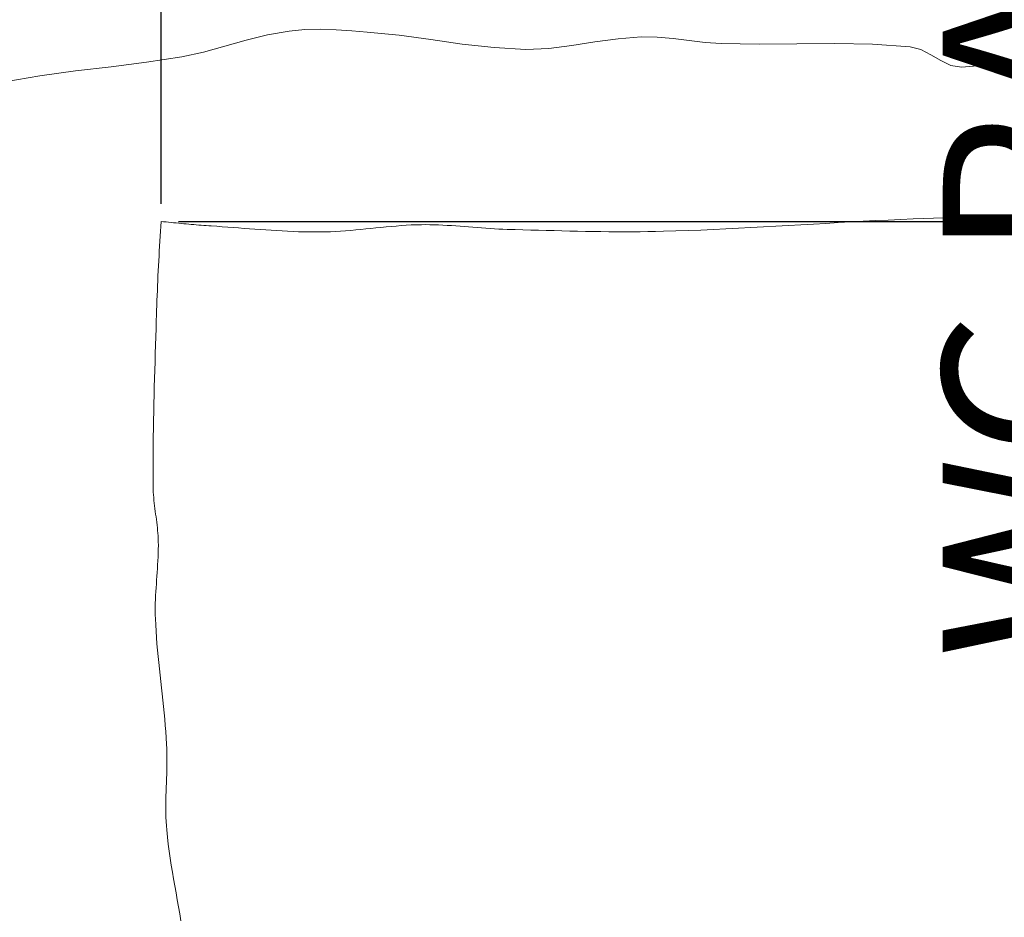
# Model space of a CAD drawing. Units: inches. Extents: x 2656 to 9931, y 1941 to 3068.
# Tile 19 of 46: x 2896 to 2932, y 2498 to 2530. Entities that reach past the tile are written whole.
import ezdxf

# ---------------------------------------------------------------- set-up
doc = ezdxf.new("R2010")
doc.units = ezdxf.units.IN
doc.layers.add('A-ANNO-DIMS', color=2, linetype='Continuous', lineweight=18)
doc.layers.add('A-FURN', color=8, linetype='Continuous', lineweight=13)
doc.styles.get("Standard").update_dxf_attribs({"font": 'arial.ttf'})
doc.dimstyles.new('ISO-25', dxfattribs={"dimtxt": 6, "dimasz": 2.5, "dimexe": 1.25, "dimexo": 0.625, "dimtad": 1, "dimdec": 0, "dimlunit": 3, "dimtxsty": 'Standard', "dimcen": 2.5, "dimadec": 0, "dimazin": 0, "dimtfac": 1, "dimtdec": 0, "dimtmove": 0, "dimatfit": 3, "dimfxl": 1, "dimarcsym": 0})

# ---------------------------------------------------------------- blocks, each defined once
blk = doc.blocks.new('BED-DOUBLE')
for p, q in [((27.981, 62.21), (27.218, 62.019)), ((28.754, 62.35), (27.981, 62.21)), ((29.308, 62.401), (28.754, 62.35)), ((29.865, 62.411), (29.308, 62.401)), ((30.423, 62.394), (29.865, 62.411)), ((30.981, 62.358), (30.423, 62.394)), ((31.538, 62.315), (30.981, 62.358)), ((32.669, 62.198), (31.538, 62.315)), ((33.797, 62.044), (32.669, 62.198)), ((41.299, 62.14), (40.475, 62.076)), ((41.872, 62.129), (41.299, 62.14)), ((42.443, 62.078), (41.872, 62.129)), ((26.459, 61.805), (25.698, 61.6)), ((27.218, 62.019), (26.459, 61.805)), ((34.924, 61.887), (33.797, 62.044)), ((36.054, 61.76), (34.924, 61.887)), ((38.833, 61.831), (38.012, 61.729)), ((39.653, 61.96), (38.833, 61.831)), ((40.475, 62.076), (39.653, 61.96)), ((43.013, 62.008), (42.443, 62.078)), ((43.584, 61.942), (43.013, 62.008)), ((44.157, 61.901), (43.584, 61.942)), ((45.504, 61.879), (44.157, 61.901)), ((46.854, 61.889), (45.504, 61.879)), ((48.203, 61.9), (46.854, 61.889)), ((49.55, 61.878), (48.203, 61.9)), ((50.893, 61.79), (49.55, 61.878)), ((51.27, 61.688), (50.893, 61.79)), ((24.929, 61.432), (23.668, 61.237)), ((25.698, 61.6), (24.929, 61.432)), ((37.187, 61.697), (36.054, 61.76)), ((38.012, 61.729), (37.187, 61.697)), ((51.627, 61.503), (51.27, 61.688)), ((51.978, 61.295), (51.627, 61.503)), ((22.401, 61.078), (21.133, 60.928)), ((23.668, 61.237), (22.401, 61.078)), ((52.336, 61.127), (51.978, 61.295)), ((52.714, 61.061), (52.336, 61.127)), ((53.7, 61.143), (52.714, 61.061)), ((54.677, 61.321), (53.7, 61.143)), ((19.868, 60.758), (18.612, 60.54)), ((21.133, 60.928), (19.868, 60.758)), ((24.187, 55.565), (24.175, 55.389)), ((24.276, 55.555), (24.187, 55.565)), ((24.366, 55.545), (24.276, 55.555)), ((24.455, 55.535), (24.366, 55.545)), ((24.544, 55.526), (24.455, 55.535)), ((24.634, 55.517), (24.544, 55.526)), ((24.723, 55.508), (24.634, 55.517)), ((24.813, 55.499), (24.723, 55.508)), ((24.902, 55.49), (24.813, 55.499)), ((24.992, 55.482), (24.902, 55.49)), ((25.081, 55.473), (24.992, 55.482)), ((25.171, 55.465), (25.081, 55.473)), ((25.26, 55.457), (25.171, 55.465)), ((47.438, 55.469), (46.993, 55.443)), ((47.883, 55.495), (47.438, 55.469)), ((48.328, 55.521), (47.883, 55.495)), ((48.773, 55.545), (48.328, 55.521)), ((49.218, 55.569), (48.773, 55.545)), ((49.663, 55.592), (49.218, 55.569)), ((50.109, 55.613), (49.663, 55.592)), ((50.554, 55.633), (50.109, 55.613)), ((50.999, 55.651), (50.554, 55.633)), ((51.36, 55.665), (50.999, 55.651)), ((51.72, 55.679), (51.36, 55.665)), ((52.081, 55.693), (51.72, 55.679)), ((52.441, 55.706), (52.081, 55.693)), ((52.802, 55.72), (52.441, 55.706)), ((53.162, 55.733), (52.802, 55.72)), ((53.522, 55.745), (53.162, 55.733)), ((53.883, 55.757), (53.522, 55.745)), ((54.244, 55.769), (53.883, 55.757)), ((54.604, 55.779), (54.244, 55.769)), ((24.164, 55.213), (24.153, 55.037)), ((24.175, 55.389), (24.164, 55.213)), ((25.35, 55.45), (25.26, 55.457)), ((25.439, 55.442), (25.35, 55.45)), ((25.529, 55.435), (25.439, 55.442)), ((25.619, 55.428), (25.529, 55.435)), ((25.708, 55.422), (25.619, 55.428)), ((25.798, 55.415), (25.708, 55.422)), ((25.888, 55.409), (25.798, 55.415)), ((25.977, 55.403), (25.888, 55.409)), ((26.172, 55.39), (25.977, 55.403)), ((26.366, 55.376), (26.172, 55.39)), ((26.56, 55.361), (26.366, 55.376)), ((26.754, 55.347), (26.56, 55.361)), ((26.949, 55.332), (26.754, 55.347)), ((27.143, 55.317), (26.949, 55.332)), ((27.337, 55.302), (27.143, 55.317)), ((27.531, 55.288), (27.337, 55.302)), ((27.726, 55.274), (27.531, 55.288)), ((27.92, 55.26), (27.726, 55.274)), ((28.114, 55.248), (27.92, 55.26)), ((28.309, 55.236), (28.114, 55.248)), ((28.503, 55.225), (28.309, 55.236)), ((28.698, 55.215), (28.503, 55.225)), ((28.892, 55.206), (28.698, 55.215)), ((29.087, 55.199), (28.892, 55.206)), ((29.281, 55.194), (29.087, 55.199)), ((29.476, 55.19), (29.281, 55.194)), ((29.67, 55.188), (29.476, 55.19)), ((29.865, 55.188), (29.67, 55.188)), ((30.045, 55.191), (29.865, 55.188)), ((30.226, 55.197), (30.045, 55.191)), ((30.406, 55.205), (30.226, 55.197)), ((30.586, 55.216), (30.406, 55.205)), ((30.766, 55.229), (30.586, 55.216)), ((30.946, 55.244), (30.766, 55.229)), ((31.126, 55.261), (30.946, 55.244)), ((31.306, 55.278), (31.126, 55.261)), ((31.486, 55.296), (31.306, 55.278)), ((31.665, 55.314), (31.486, 55.296)), ((31.845, 55.333), (31.665, 55.314)), ((32.025, 55.351), (31.845, 55.333)), ((32.205, 55.369), (32.025, 55.351)), ((32.385, 55.386), (32.205, 55.369)), ((32.565, 55.401), (32.385, 55.386)), ((32.745, 55.415), (32.565, 55.401)), ((32.925, 55.427), (32.745, 55.415)), ((33.105, 55.437), (32.925, 55.427)), ((33.285, 55.444), (33.105, 55.437)), ((33.466, 55.448), (33.285, 55.444)), ((33.619, 55.449), (33.466, 55.448)), ((33.772, 55.447), (33.619, 55.449)), ((33.926, 55.444), (33.772, 55.447)), ((34.079, 55.439), (33.926, 55.444)), ((34.232, 55.432), (34.079, 55.439)), ((34.385, 55.424), (34.232, 55.432)), ((34.538, 55.414), (34.385, 55.424)), ((34.691, 55.404), (34.538, 55.414)), ((34.844, 55.392), (34.691, 55.404)), ((34.997, 55.381), (34.844, 55.392)), ((35.15, 55.369), (34.997, 55.381)), ((35.303, 55.356), (35.15, 55.369)), ((35.456, 55.344), (35.303, 55.356)), ((35.609, 55.333), (35.456, 55.344)), ((35.762, 55.322), (35.609, 55.333)), ((35.915, 55.311), (35.762, 55.322)), ((36.068, 55.302), (35.915, 55.311)), ((36.221, 55.294), (36.068, 55.302)), ((36.374, 55.287), (36.221, 55.294)), ((36.528, 55.282), (36.374, 55.287)), ((36.806, 55.274), (36.528, 55.282)), ((37.084, 55.266), (36.806, 55.274)), ((37.362, 55.258), (37.084, 55.266)), ((37.641, 55.25), (37.362, 55.258)), ((37.919, 55.243), (37.641, 55.25)), ((38.198, 55.235), (37.919, 55.243)), ((38.476, 55.228), (38.198, 55.235)), ((38.754, 55.221), (38.476, 55.228)), ((39.033, 55.215), (38.754, 55.221)), ((39.311, 55.21), (39.033, 55.215)), ((39.59, 55.205), (39.311, 55.21)), ((39.868, 55.201), (39.59, 55.205)), ((40.146, 55.198), (39.868, 55.201)), ((40.425, 55.196), (40.146, 55.198)), ((40.703, 55.195), (40.425, 55.196)), ((40.982, 55.196), (40.703, 55.195)), ((41.26, 55.197), (40.982, 55.196)), ((41.538, 55.2), (41.26, 55.197)), ((41.817, 55.205), (41.538, 55.2)), ((42.095, 55.211), (41.817, 55.205)), ((42.54, 55.224), (42.095, 55.211)), ((42.986, 55.239), (42.54, 55.224)), ((43.431, 55.256), (42.986, 55.239)), ((43.877, 55.275), (43.431, 55.256)), ((44.322, 55.296), (43.877, 55.275)), ((44.767, 55.318), (44.322, 55.296)), ((45.212, 55.342), (44.767, 55.318)), ((45.657, 55.366), (45.212, 55.342)), ((46.103, 55.391), (45.657, 55.366)), ((46.548, 55.417), (46.103, 55.391)), ((46.993, 55.443), (46.548, 55.417)), ((24.142, 54.861), (24.132, 54.685)), ((24.153, 55.037), (24.142, 54.861)), ((24.122, 54.508), (24.112, 54.332)), ((24.132, 54.685), (24.122, 54.508)), ((24.103, 54.156), (24.093, 53.98)), ((24.112, 54.332), (24.103, 54.156)), ((24.085, 53.803), (24.076, 53.627)), ((24.093, 53.98), (24.085, 53.803)), ((24.068, 53.451), (24.06, 53.274)), ((24.076, 53.627), (24.068, 53.451)), ((24.053, 53.098), (24.046, 52.922)), ((24.06, 53.274), (24.053, 53.098)), ((24.039, 52.745), (24.033, 52.569)), ((24.046, 52.922), (24.039, 52.745)), ((24.026, 52.393), (24.021, 52.216)), ((24.033, 52.569), (24.026, 52.393)), ((24.015, 52.04), (24.006, 51.743)), ((24.021, 52.216), (24.015, 52.04)), ((24.006, 51.743), (23.997, 51.447)), ((23.997, 51.447), (23.988, 51.151)), ((23.988, 51.151), (23.979, 50.854)), ((23.97, 50.558), (23.961, 50.261)), ((23.979, 50.854), (23.97, 50.558)), ((23.961, 50.261), (23.953, 49.965)), ((23.953, 49.965), (23.944, 49.668)), ((23.944, 49.668), (23.937, 49.372)), ((23.937, 49.372), (23.929, 49.076)), ((23.929, 49.076), (23.923, 48.779)), ((23.917, 48.483), (23.912, 48.186)), ((23.923, 48.779), (23.917, 48.483)), ((23.912, 48.186), (23.907, 47.89)), ((23.907, 47.89), (23.904, 47.593)), ((23.904, 47.593), (23.901, 47.297)), ((23.901, 47.297), (23.899, 47)), ((23.899, 47), (23.899, 46.704)), ((23.899, 46.704), (23.9, 46.407)), ((23.9, 46.407), (23.902, 46.111)), ((23.902, 46.111), (23.904, 46.013)), ((23.904, 46.013), (23.908, 45.915)), ((23.908, 45.915), (23.914, 45.817)), ((23.914, 45.817), (23.922, 45.719)), ((23.922, 45.719), (23.932, 45.621)), ((23.932, 45.621), (23.942, 45.524)), ((23.942, 45.524), (23.954, 45.426)), ((23.954, 45.426), (23.966, 45.329)), ((23.966, 45.329), (23.979, 45.231)), ((23.979, 45.231), (23.992, 45.134)), ((23.992, 45.134), (24.006, 45.036)), ((24.006, 45.036), (24.019, 44.939)), ((24.019, 44.939), (24.031, 44.841)), ((24.031, 44.841), (24.043, 44.744)), ((24.043, 44.744), (24.054, 44.646)), ((24.054, 44.646), (24.064, 44.548)), ((24.064, 44.548), (24.072, 44.451)), ((24.072, 44.451), (24.079, 44.353)), ((24.079, 44.353), (24.084, 44.255)), ((24.084, 44.255), (24.087, 44.157)), ((24.087, 43.882), (24.083, 43.744)), ((24.087, 44.157), (24.088, 44.019)), ((24.088, 44.019), (24.087, 43.882)), ((24.078, 43.606), (24.072, 43.469)), ((24.083, 43.744), (24.078, 43.606)), ((24.055, 43.194), (24.046, 43.056)), ((24.064, 43.331), (24.055, 43.194)), ((24.072, 43.469), (24.064, 43.331)), ((24.036, 42.919), (24.026, 42.781)), ((24.046, 43.056), (24.036, 42.919)), ((24.007, 42.506), (23.999, 42.369)), ((24.017, 42.644), (24.007, 42.506)), ((24.026, 42.781), (24.017, 42.644)), ((23.991, 42.231), (23.985, 42.094)), ((23.999, 42.369), (23.991, 42.231)), ((23.977, 41.818), (23.976, 41.681)), ((23.98, 41.956), (23.977, 41.818)), ((23.985, 42.094), (23.98, 41.956)), ((23.976, 41.681), (23.978, 41.543)), ((23.978, 41.543), (23.982, 41.406)), ((23.982, 41.406), (23.993, 41.182)), ((23.993, 41.182), (24.006, 40.957)), ((24.006, 40.957), (24.022, 40.734)), ((24.022, 40.734), (24.04, 40.51)), ((24.04, 40.51), (24.059, 40.286)), ((24.059, 40.286), (24.08, 40.062)), ((24.08, 40.062), (24.103, 39.839)), ((24.103, 39.839), (24.126, 39.615)), ((24.126, 39.615), (24.151, 39.392)), ((24.151, 39.392), (24.175, 39.169)), ((24.175, 39.169), (24.2, 38.945)), ((24.2, 38.945), (24.225, 38.722)), ((24.225, 38.722), (24.249, 38.499)), ((24.249, 38.499), (24.272, 38.275)), ((24.272, 38.275), (24.295, 38.052)), ((24.295, 38.052), (24.316, 37.828)), ((24.316, 37.828), (24.336, 37.604)), ((24.336, 37.604), (24.354, 37.38)), ((24.354, 37.38), (24.37, 37.156)), ((24.37, 37.156), (24.383, 36.932)), ((24.383, 36.932), (24.39, 36.78)), ((24.39, 36.78), (24.394, 36.627)), ((24.394, 36.627), (24.396, 36.474)), ((24.394, 36.168), (24.39, 36.015)), ((24.395, 36.321), (24.394, 36.168)), ((24.396, 36.474), (24.395, 36.321)), ((24.386, 35.862), (24.381, 35.709)), ((24.39, 36.015), (24.386, 35.862)), ((24.376, 35.555), (24.37, 35.402)), ((24.381, 35.709), (24.376, 35.555)), ((24.365, 35.249), (24.361, 35.096)), ((24.37, 35.402), (24.365, 35.249)), ((24.358, 34.943), (24.355, 34.79)), ((24.355, 34.79), (24.355, 34.637)), ((24.361, 35.096), (24.358, 34.943)), ((24.355, 34.637), (24.356, 34.485)), ((24.356, 34.485), (24.36, 34.332)), ((24.36, 34.332), (24.367, 34.179)), ((24.367, 34.179), (24.376, 34.027)), ((24.376, 34.027), (24.389, 33.875)), ((24.389, 33.875), (24.415, 33.624)), ((24.415, 33.624), (24.444, 33.374)), ((24.444, 33.374), (24.477, 33.124)), ((24.477, 33.124), (24.512, 32.875)), ((24.512, 32.875), (24.55, 32.626)), ((24.55, 32.626), (24.59, 32.377)), ((24.59, 32.377), (24.632, 32.129)), ((24.632, 32.129), (24.675, 31.881)), ((24.675, 31.881), (24.719, 31.632)), ((24.719, 31.632), (24.763, 31.384)), ((24.763, 31.384), (24.808, 31.136)), ((24.808, 31.136), (24.852, 30.888)), ((24.852, 30.888), (24.895, 30.639))]:
    blk.add_line(p, q)
blk = doc.blocks.new('*D29')
at = {"layer": 'A-ANNO-DIMS', "color": 0, "lineweight": -2, "transparency": 16777216}
for p, q in [((2939.241, 2614.856), (2935.66, 2614.856)), ((2936.91, 2612.356), (2936.91, 2597.652)), ((2939.241, 2595.152), (2935.66, 2595.152)), ((2936.91, 2595.152), (2936.91, 2504.746))]:
    blk.add_line(p, q, dxfattribs=at)
at = {"layer": 'A-ANNO-DIMS', "color": 0, "transparency": 16777216}
for points in [[(2936.493, 2612.356), (2937.327, 2612.356), (2936.91, 2614.856)], [(2936.493, 2597.652), (2937.327, 2597.652), (2936.91, 2595.152)]]:
    blk.add_solid(points, dxfattribs=at)
at = {"layer": 'Defpoints', "color": 0, "transparency": 16777216}
for p in [(2939.866, 2614.856), (2936.91, 2595.152), (2939.866, 2595.152)]:
    blk.add_point(p, dxfattribs=at)
at = {"layer": 'A-ANNO-DIMS', "color": 0, "transparency": 16777216, "insert": (2933.183, 2548.699), "char_height": 6, "attachment_point": 5, "rotation": 90}
blk.add_mtext('WC PAN 1\'-7 1/2" TYP.', dxfattribs=at)
blk = doc.blocks.new('*D31')
at = {"layer": 'A-ANNO-DIMS', "color": 0, "lineweight": -2, "transparency": 16777216}
for p, q in [((2753.358, 2502.145), (2753.358, 2488.227)), ((2841.982, 2502.145), (2841.982, 2488.227)), ((2755.858, 2489.477), (2839.482, 2489.477)), ((2841.982, 2489.477), (2952.348, 2489.477))]:
    blk.add_line(p, q, dxfattribs=at)
at = {"layer": 'A-ANNO-DIMS', "color": 0, "transparency": 16777216}
for points in [[(2755.858, 2489.893), (2755.858, 2489.06), (2753.358, 2489.477)], [(2839.482, 2489.893), (2839.482, 2489.06), (2841.982, 2489.477)]]:
    blk.add_solid(points, dxfattribs=at)
at = {"layer": 'Defpoints', "color": 0, "transparency": 16777216}
for p in [(2753.358, 2502.77), (2841.982, 2502.77), (2841.982, 2489.477)]:
    blk.add_point(p, dxfattribs=at)
at = {"layer": 'A-ANNO-DIMS', "color": 0, "transparency": 16777216, "insert": (2898.415, 2493.206), "char_height": 6, "attachment_point": 5}
blk.add_mtext('DOUBLE BED 7\'-4 1/2" TYP.', dxfattribs=at)
blk = doc.blocks.new('*D102')
at = {"layer": 'A-ANNO-DIMS', "color": 0, "lineweight": -2, "transparency": 16777216}
for p, q in [((2998.157, 2604.975), (2998.157, 2009.273)), ((2872.157, 2564.712), (2872.157, 2009.273)), ((2874.657, 2010.523), (2995.657, 2010.523))]:
    blk.add_line(p, q, dxfattribs=at)
at = {"layer": 'A-ANNO-DIMS', "color": 0, "transparency": 16777216}
for points in [[(2874.657, 2010.939), (2874.657, 2010.106), (2872.157, 2010.523)], [(2995.657, 2010.939), (2995.657, 2010.106), (2998.157, 2010.523)]]:
    blk.add_solid(points, dxfattribs=at)
at = {"layer": 'Defpoints', "color": 0, "transparency": 16777216}
for p in [(2998.157, 2605.6), (2872.157, 2565.337), (2998.157, 2010.523)]:
    blk.add_point(p, dxfattribs=at)
at = {"layer": 'A-ANNO-DIMS', "color": 0, "transparency": 16777216, "insert": (2935.157, 2014.211), "char_height": 6, "attachment_point": 5}
blk.add_mtext('10\'-6"', dxfattribs=at)
blk = doc.blocks.new('*D130')
at = {"layer": 'A-ANNO-DIMS', "color": 0, "lineweight": -2, "transparency": 16777216}
for p, q in [((2877.282, 2538.52), (3061.007, 2538.52)), ((3059.757, 2536.02), (3059.757, 2525.316)), ((2902.165, 2522.816), (3061.007, 2522.816)), ((3059.757, 2522.816), (3059.757, 2489.7))]:
    blk.add_line(p, q, dxfattribs=at)
at = {"layer": 'A-ANNO-DIMS', "color": 0, "transparency": 16777216}
for points in [[(3059.341, 2536.02), (3060.174, 2536.02), (3059.757, 2538.52)], [(3059.341, 2525.316), (3060.174, 2525.316), (3059.757, 2522.816)]]:
    blk.add_solid(points, dxfattribs=at)
at = {"layer": 'Defpoints', "color": 0, "transparency": 16777216}
for p in [(2876.657, 2538.52), (2901.54, 2522.816), (3059.757, 2522.816)]:
    blk.add_point(p, dxfattribs=at)
at = {"layer": 'A-ANNO-DIMS', "color": 0, "transparency": 16777216, "insert": (3056.028, 2505.008), "char_height": 6, "attachment_point": 5, "rotation": 90}
blk.add_mtext('1\'-3 1/2"', dxfattribs=at)
blk = doc.blocks.new('*D131')
at = {"layer": 'A-ANNO-DIMS', "color": 0, "lineweight": -2, "transparency": 16777216}
for p, q in [((2876.657, 2539.145), (2876.657, 2674.45)), ((2901.54, 2523.441), (2901.54, 2674.45)), ((2879.157, 2673.2), (2899.04, 2673.2))]:
    blk.add_line(p, q, dxfattribs=at)
at = {"layer": 'A-ANNO-DIMS', "color": 0, "transparency": 16777216}
for points in [[(2879.157, 2673.617), (2879.157, 2672.784), (2876.657, 2673.2)], [(2899.04, 2673.617), (2899.04, 2672.784), (2901.54, 2673.2)]]:
    blk.add_solid(points, dxfattribs=at)
at = {"layer": 'Defpoints', "color": 0, "transparency": 16777216}
for p in [(2901.54, 2673.2), (2876.657, 2538.52), (2901.54, 2522.816)]:
    blk.add_point(p, dxfattribs=at)
at = {"layer": 'A-ANNO-DIMS', "color": 0, "transparency": 16777216, "insert": (2889.099, 2676.838), "char_height": 6, "attachment_point": 5}
blk.add_mtext('2\'-1"', dxfattribs=at)

msp = doc.modelspace()

# ---------------------------------------------------------------- block references
at = {"layer": 'A-FURN'}
msp.add_blockref('BED-DOUBLE', (2877.353, 2467.251), dxfattribs=at)

# ---------------------------------------------------------------- dimensions: what is measured, and where the dimension line sits
at = {"layer": 'A-ANNO-DIMS'}
for base, p1, p2, picture, middle in [((2901.54, 2673.2), (2876.657, 2538.52), (2901.54, 2522.816), '*D131', (2889.099, 2676.838)), ((2998.157, 2010.523), (2872.157, 2565.337), (2998.157, 2605.6), '*D102', (2935.157, 2014.211))]:
    dim = msp.add_linear_dim(base=base, p1=p1, p2=p2, dimstyle='ISO-25', override={"dimdec": 1, "dimlfac": 1, "dimrnd": 0, "dimzin": 1, "dimdsep": 46, "dimlunit": 4, "dimfrac": 2}, dxfattribs=at)
    dim.commit()
    dim.dimension.update_dxf_attribs({"geometry": picture, "text_midpoint": middle})
dim = msp.add_linear_dim(base=(2936.91, 2595.152), p1=(2939.866, 2614.856), p2=(2939.866, 2595.152), angle=270, text='WC PAN <> TYP.', dimstyle='ISO-25', override={"dimdec": 1, "dimlfac": 1, "dimrnd": 0, "dimzin": 1, "dimdsep": 46, "dimlunit": 4, "dimfrac": 2}, dxfattribs=at)
dim.commit()
dim.dimension.update_dxf_attribs({"geometry": '*D29', "text_midpoint": (2933.183, 2548.699)})
dim = msp.add_linear_dim(base=(3059.757, 2522.816), p1=(2876.657, 2538.52), p2=(2901.54, 2522.816), angle=90, dimstyle='ISO-25', override={"dimdec": 1, "dimlfac": 1, "dimrnd": 0, "dimzin": 1, "dimdsep": 46, "dimlunit": 4, "dimfrac": 2}, dxfattribs=at)
dim.commit()
dim.dimension.update_dxf_attribs({"geometry": '*D130', "text_midpoint": (3056.028, 2505.008)})
dim = msp.add_linear_dim(base=(2841.982, 2489.477), p1=(2753.358, 2502.77), p2=(2841.982, 2502.77), text='DOUBLE BED <> TYP.', dimstyle='ISO-25', override={"dimdec": 1, "dimlfac": 1, "dimrnd": 0, "dimzin": 1, "dimdsep": 46, "dimlunit": 4, "dimfrac": 2}, dxfattribs=at)
dim.commit()
dim.dimension.update_dxf_attribs({"geometry": '*D31', "text_midpoint": (2898.415, 2493.206)})

doc.saveas('drawing.dxf')
